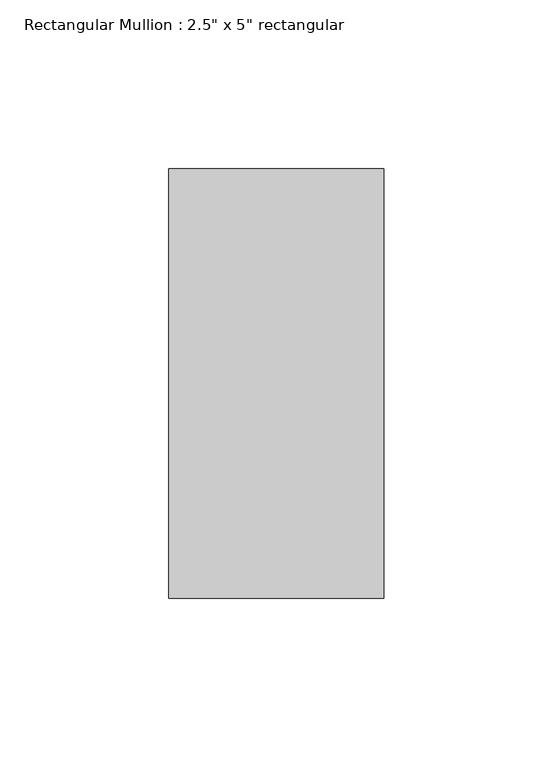
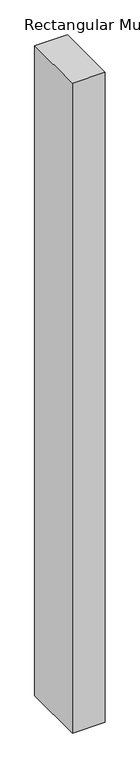
"""IFC4 building model written with IfcOpenShell, lengths in millimetres: member geometry."""

from ifc_helpers import new_model, si_unit, frame, origin, place, context, project, spatial, polyline, outline, extrude, source, transform, mapped, element, save


def member_afc9459e(model_context):
    return source(origin(), model_context, "Body", "SweptSolid", [
        extrude(outline(polyline([(31.75, 63.5), (31.75, -63.5), (-31.75, -63.5), (-31.75, 63.5), (31.75, 63.5)])), frame((0.0, 0.0, -1333.5), z_axis=(0.0, 0.0, 1.0), x_axis=(1.0, 0.0, 0.0)), (0.0, 0.0, 1.0), 1333.5),
    ])


if __name__ == "__main__":
    model = new_model("IFC4")
    model_context = context("Model", 3, world=origin())
    ifc_project = project(units=[si_unit("LENGTHUNIT", "METRE", prefix="MILLI")], contexts=[model_context])
    site = spatial("IfcSite", under=ifc_project)
    building = spatial("IfcBuilding", under=site)
    placement = place(None, origin())
    member_shape = member_afc9459e(model_context)
    element("IfcMember", 1, ObjectType="Rectangular Mullion : 2.5\" x 5\" rectangular", at=placement, inside=building, context=model_context, shape_type="MappedRepresentation", body=[
        mapped(member_shape, transform((0.0, 0.0, 0.0), x_axis=(1.0, 0.0, 0.0), y_axis=(0.0, 1.0, 0.0), z_axis=(0.0, 0.0, 1.0))),
    ])
    save(model, "model.ifc")

# Revit data of these elements
# Type "Rectangular Mullion : 2.5\" x 5\" rectangular"
#   built-in parameter 1007304 = 0.416667 (stored number, unit not read)
#   built-in parameter 1007301 = 0.104167 (stored number, unit not read)
#   built-in parameter 1007300 = 0.104167 (stored number, unit not read)
# Element 1 (IfcMember, "Rectangular Mullion : 2.5\" x 5\" rectangular")
#   Materials on its faces: "Aluminum"
# Materials
#   "Aluminum": class "Metal", colour RGB 247 247 247, transparency 0, Description = "Aluminum 6061", Cost = 0
